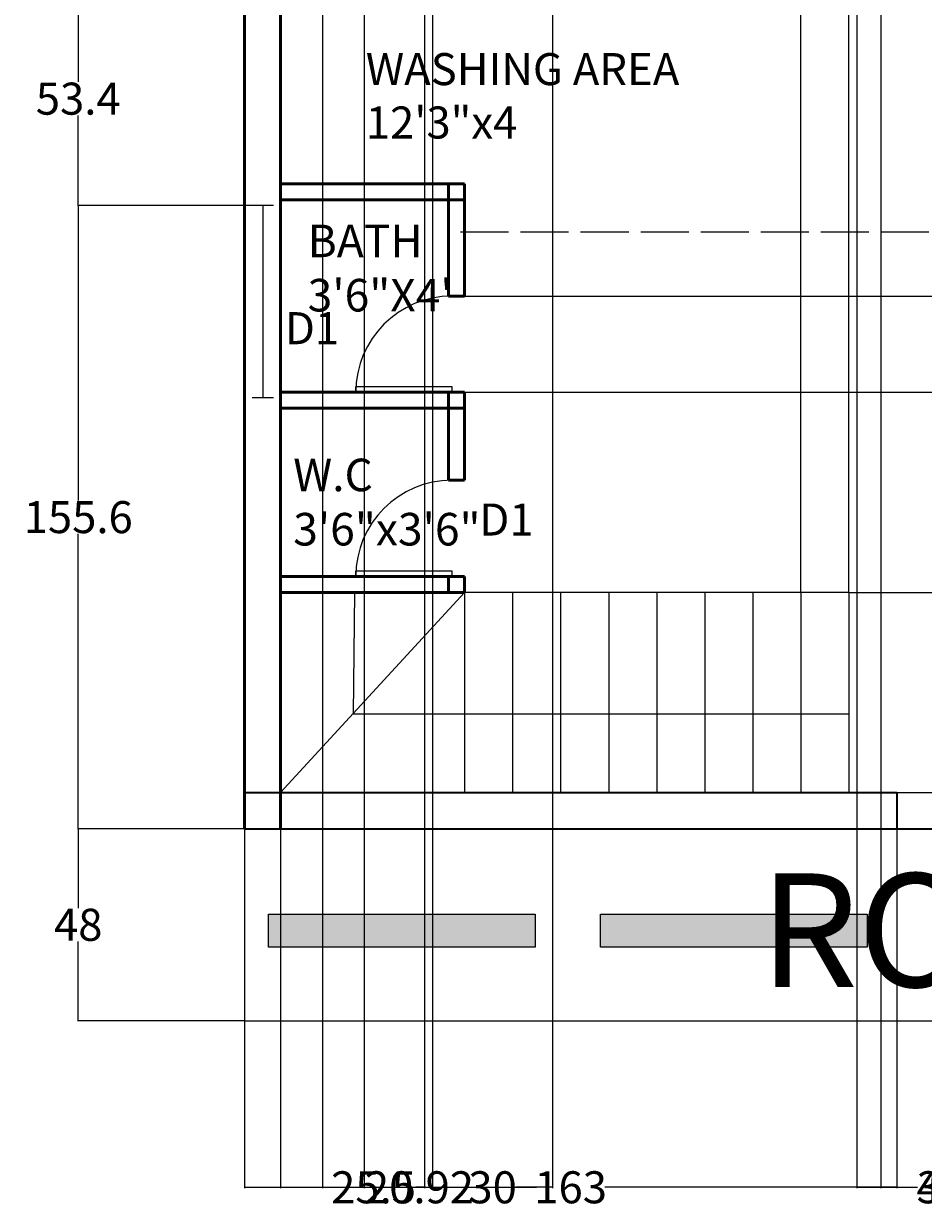
# Model space of a CAD drawing. Units: inches. Extents: x 3004 to 3478, y -798 to 114.
# Tile 1 of 5: x 3007 to 3232, y -798 to -503. Entities that reach past the tile are written whole.
import ezdxf

# ---------------------------------------------------------------- set-up
doc = ezdxf.new("R2010")
doc.units = ezdxf.units.IN
doc.header["$MEASUREMENT"] = 0
doc.linetypes.add('ACAD_ISO02W100', pattern=[15, 12, -3])
for name, color, linetype, lineweight in [('A-ANNO-DIMS', 2, 'Continuous', 18), ('A-ANNO-TEXT', 7, 'Continuous', 18), ('A-AREA-IDEN', 7, 'Continuous', 18), ('A-DOOR', 4, 'Continuous', 25), ('A-FLOR-OVHD', 8, 'ACAD_ISO02W100', 18), ('A-FLOR-STRS', 7, 'Continuous', 25), ('A-GLAZ', 4, 'Continuous', 25), ('A-WALL', 7, 'Continuous', 50), ('A-WALL-SITE', 7, 'Continuous', 35), ('C-ROAD', 8, 'Continuous', 25), ('C-ROAD-MARK', 8, 'Continuous', 18), ('C-ROAD-PATT', 8, 'Continuous', 13)]:
    doc.layers.add(name, color=color, linetype=linetype, lineweight=lineweight)
doc.styles.get("Standard").update_dxf_attribs({"font": 'arial.ttf', "height": 8})
doc.dimstyles.get("Standard").update_dxf_attribs({"dimtxt": 0.18, "dimasz": 0.18, "dimexe": 0.18, "dimexo": 0.0625, "dimgap": 0.09, "dimtad": 0, "dimtih": 1, "dimtoh": 1, "dimzin": 0, "dimdsep": 46, "dimlunit": 4, "dimtxsty": 'Standard', "dimcen": 0.09, "dimadec": 0, "dimazin": 0, "dimtfac": 1, "dimtofl": 0, "dimtmove": 0, "dimatfit": 3, "dimfxl": 1, "dimtolj": 1, "dimtzin": 0, "dimarcsym": 0})

# ---------------------------------------------------------------- blocks, each defined once
blk = doc.blocks.new('*U19')
for p, q in [((0, 0), (0, -100)), ((750, 0), (750, -100))]:
    blk.add_line(p, q)
blk.add_lwpolyline([(0, 0), (0, 750), (43.75, 750), (43.75, 0)], close=True)
blk.add_arc((0, 0), 750, 0, 90)
blk = doc.blocks.new('Window - Imperial')
for p, q in [((0, 4), (0, 0)), ((36, 4), (36, 0)), ((0, 2), (36, 2))]:
    blk.add_line(p, q)
blk = doc.blocks.new('*D40')
at = {"layer": 'A-ANNO-DIMS', "color": 0, "lineweight": -2, "transparency": 16777216}
for p, q in [((3064.06, -548.08), (3020.48, -548.08)), ((3020.66, -548.26), (3020.66, -621.71)), ((3020.66, -703.5), (3020.66, -630.05)), ((3062.15, -703.68), (3020.48, -703.68))]:
    blk.add_line(p, q, dxfattribs=at)
at = {"layer": 'A-ANNO-DIMS', "color": 0, "transparency": 16777216}
for points in [[(3020.63, -548.26), (3020.69, -548.26), (3020.66, -548.08)], [(3020.63, -703.5), (3020.69, -703.5), (3020.66, -703.68)]]:
    blk.add_solid(points, dxfattribs=at)
at = {"layer": 'Defpoints', "color": 0, "transparency": 16777216}
for p in [(3064.12, -548.08), (3020.66, -703.68), (3062.21, -703.68)]:
    blk.add_point(p, dxfattribs=at)
at = {"layer": 'A-ANNO-DIMS', "color": 0, "transparency": 16777216, "insert": (3020.66, -625.88), "char_height": 8, "attachment_point": 5}
blk.add_mtext('\\A1;155.6', dxfattribs=at)
blk = doc.blocks.new('*D41')
at = {"layer": 'A-ANNO-DIMS', "color": 0, "lineweight": -2, "transparency": 16777216}
for p, q in [((3062.15, -703.68), (3020.48, -703.68)), ((3020.66, -703.86), (3020.66, -723.5)), ((3020.66, -751.5), (3020.66, -731.85)), ((3062.15, -751.68), (3020.48, -751.68))]:
    blk.add_line(p, q, dxfattribs=at)
at = {"layer": 'A-ANNO-DIMS', "color": 0, "transparency": 16777216}
for points in [[(3020.63, -703.86), (3020.69, -703.86), (3020.66, -703.68)], [(3020.63, -751.5), (3020.69, -751.5), (3020.66, -751.68)]]:
    blk.add_solid(points, dxfattribs=at)
at = {"layer": 'Defpoints', "color": 0, "transparency": 16777216}
for p in [(3062.21, -703.68), (3020.66, -751.68), (3062.21, -751.68)]:
    blk.add_point(p, dxfattribs=at)
at = {"layer": 'A-ANNO-DIMS', "color": 0, "transparency": 16777216, "insert": (3020.66, -727.68), "char_height": 8, "attachment_point": 5}
blk.add_mtext('\\A1;48', dxfattribs=at)
blk = doc.blocks.new('*D42')
at = {"layer": 'A-ANNO-DIMS', "color": 0, "lineweight": -2, "transparency": 16777216}
for p, q in [((3062.21, -703.74), (3062.21, -793.41)), ((3225.21, -703.74), (3225.21, -793.41)), ((3062.39, -793.23), (3135.16, -793.23)), ((3225.03, -793.23), (3152.26, -793.23))]:
    blk.add_line(p, q, dxfattribs=at)
at = {"layer": 'A-ANNO-DIMS', "color": 0, "transparency": 16777216}
for points in [[(3062.39, -793.2), (3062.39, -793.26), (3062.21, -793.23)], [(3225.03, -793.2), (3225.03, -793.26), (3225.21, -793.23)]]:
    blk.add_solid(points, dxfattribs=at)
at = {"layer": 'Defpoints', "color": 0, "transparency": 16777216}
for p in [(3062.21, -703.68), (3225.21, -703.68), (3225.21, -793.23)]:
    blk.add_point(p, dxfattribs=at)
at = {"layer": 'A-ANNO-DIMS', "color": 0, "transparency": 16777216, "insert": (3143.71, -793.23), "char_height": 8, "attachment_point": 5}
blk.add_mtext('\\A1;163', dxfattribs=at)
blk = doc.blocks.new('*D52')
at = {"layer": 'A-ANNO-DIMS', "color": 0, "lineweight": -2, "transparency": 16777216}
for p, q in [((3071.15, -494.68), (3020.48, -494.68)), ((3020.66, -494.86), (3020.66, -517.2)), ((3020.66, -547.9), (3020.66, -525.56)), ((3064.06, -548.08), (3020.48, -548.08))]:
    blk.add_line(p, q, dxfattribs=at)
at = {"layer": 'A-ANNO-DIMS', "color": 0, "transparency": 16777216}
for points in [[(3020.63, -494.86), (3020.69, -494.86), (3020.66, -494.68)], [(3020.63, -547.9), (3020.69, -547.9), (3020.66, -548.08)]]:
    blk.add_solid(points, dxfattribs=at)
at = {"layer": 'Defpoints', "color": 0, "transparency": 16777216}
for p in [(3071.21, -494.68), (3020.66, -548.08), (3064.12, -548.08)]:
    blk.add_point(p, dxfattribs=at)
at = {"layer": 'A-ANNO-DIMS', "color": 0, "transparency": 16777216, "insert": (3020.66, -521.38), "char_height": 8, "attachment_point": 5}
blk.add_mtext('\\A1;53.4', dxfattribs=at)
blk = doc.blocks.new('*D53')
at = {"layer": 'A-ANNO-DIMS', "color": 0, "lineweight": -2, "transparency": 16777216}
for p, q in [((3092.13, 11.22), (3092.13, -793.41)), ((3071.21, 7.26), (3071.21, -793.41)), ((3071.39, -793.23), (3091.95, -793.23)), ((3092.13, -793.23), (3092.31, -793.23))]:
    blk.add_line(p, q, dxfattribs=at)
at = {"layer": 'A-ANNO-DIMS', "color": 0, "transparency": 16777216}
for points in [[(3071.39, -793.2), (3071.39, -793.26), (3071.21, -793.23)], [(3091.95, -793.2), (3091.95, -793.26), (3092.13, -793.23)]]:
    blk.add_solid(points, dxfattribs=at)
at = {"layer": 'Defpoints', "color": 0, "transparency": 16777216}
for p in [(3092.13, 11.28), (3071.21, 7.32), (3092.13, -793.23)]:
    blk.add_point(p, dxfattribs=at)
at = {"layer": 'A-ANNO-DIMS', "color": 0, "transparency": 16777216, "insert": (3105.93, -793.23), "char_height": 8, "attachment_point": 5}
blk.add_mtext('\\A1;20.92', dxfattribs=at)
blk = doc.blocks.new('*D56')
at = {"layer": 'A-ANNO-DIMS', "color": 0, "lineweight": -2, "transparency": 16777216}
for p, q in [((3213.27, -644.68), (3463.94, -644.68)), ((3463.76, -644.86), (3463.76, -665.5)), ((3463.76, -694.5), (3463.76, -673.85)), ((3213.27, -694.68), (3463.94, -694.68))]:
    blk.add_line(p, q, dxfattribs=at)
at = {"layer": 'A-ANNO-DIMS', "color": 0, "transparency": 16777216}
for points in [[(3463.73, -644.86), (3463.79, -644.86), (3463.76, -644.68)], [(3463.73, -694.5), (3463.79, -694.5), (3463.76, -694.68)]]:
    blk.add_solid(points, dxfattribs=at)
at = {"layer": 'Defpoints', "color": 0, "transparency": 16777216}
for p in [(3213.21, -644.68), (3213.21, -694.68), (3463.76, -694.68)]:
    blk.add_point(p, dxfattribs=at)
at = {"layer": 'A-ANNO-DIMS', "color": 0, "transparency": 16777216, "insert": (3463.76, -669.68), "char_height": 8, "attachment_point": 5}
blk.add_mtext('\\A1;50', dxfattribs=at)
blk = doc.blocks.new('*D57')
at = {"layer": 'A-ANNO-DIMS', "color": 0, "lineweight": -2, "transparency": 16777216}
for p, q in [((3201.21, -644.62), (3201.21, 109.05)), ((3201.39, 108.87), (3201.81, 108.87)), ((3213.03, 108.87), (3212.61, 108.87)), ((3213.21, -644.62), (3213.21, 109.05))]:
    blk.add_line(p, q, dxfattribs=at)
at = {"layer": 'A-ANNO-DIMS', "color": 0, "transparency": 16777216}
for points in [[(3201.39, 108.9), (3201.39, 108.84), (3201.21, 108.87)], [(3213.03, 108.9), (3213.03, 108.84), (3213.21, 108.87)]]:
    blk.add_solid(points, dxfattribs=at)
at = {"layer": 'Defpoints', "color": 0, "transparency": 16777216}
for p in [(3213.21, 108.87), (3201.21, -644.68), (3213.21, -644.68)]:
    blk.add_point(p, dxfattribs=at)
at = {"layer": 'A-ANNO-DIMS', "color": 0, "transparency": 16777216, "insert": (3207.21, 108.87), "char_height": 8, "attachment_point": 5}
blk.add_mtext('\\A1;12', dxfattribs=at)
blk = doc.blocks.new('*D58')
at = {"layer": 'A-ANNO-DIMS', "color": 0, "lineweight": -2, "transparency": 16777216}
for p, q in [((3117.27, -570.68), (3463.94, -570.68)), ((3463.76, -570.86), (3463.76, -578.57)), ((3463.76, -594.5), (3463.76, -586.78)), ((3117.27, -594.68), (3463.94, -594.68))]:
    blk.add_line(p, q, dxfattribs=at)
at = {"layer": 'A-ANNO-DIMS', "color": 0, "transparency": 16777216}
for points in [[(3463.73, -570.86), (3463.79, -570.86), (3463.76, -570.68)], [(3463.73, -594.5), (3463.79, -594.5), (3463.76, -594.68)]]:
    blk.add_solid(points, dxfattribs=at)
at = {"layer": 'Defpoints', "color": 0, "transparency": 16777216}
for p in [(3117.21, -570.68), (3117.21, -594.68), (3463.76, -594.68)]:
    blk.add_point(p, dxfattribs=at)
at = {"layer": 'A-ANNO-DIMS', "color": 0, "transparency": 16777216, "insert": (3463.76, -582.68), "char_height": 8, "attachment_point": 5}
blk.add_mtext('\\A1;24', dxfattribs=at)
blk = doc.blocks.new('*D62')
at = {"layer": 'A-ANNO-DIMS', "color": 0, "lineweight": -2, "transparency": 16777216}
for p, q in [((3081.71, -334.74), (3081.71, -793.41)), ((3107.21, -334.74), (3107.21, -793.41)), ((3081.89, -793.23), (3083.88, -793.23)), ((3107.03, -793.23), (3105.04, -793.23))]:
    blk.add_line(p, q, dxfattribs=at)
at = {"layer": 'A-ANNO-DIMS', "color": 0, "transparency": 16777216}
for points in [[(3081.89, -793.2), (3081.89, -793.26), (3081.71, -793.23)], [(3107.03, -793.2), (3107.03, -793.26), (3107.21, -793.23)]]:
    blk.add_solid(points, dxfattribs=at)
at = {"layer": 'Defpoints', "color": 0, "transparency": 16777216}
for p in [(3081.71, -334.68), (3107.21, -334.68), (3107.21, -793.23)]:
    blk.add_point(p, dxfattribs=at)
at = {"layer": 'A-ANNO-DIMS', "color": 0, "transparency": 16777216, "insert": (3094.46, -793.23), "char_height": 8, "attachment_point": 5}
blk.add_mtext('\\A1;25.5', dxfattribs=at)
blk = doc.blocks.new('*D63')
at = {"layer": 'A-ANNO-DIMS', "color": 0, "lineweight": -2, "transparency": 16777216}
for p, q in [((3221.21, -46.74), (3221.21, -793.41)), ((3251.21, -46.74), (3251.21, -793.41)), ((3221.39, -793.23), (3230.41, -793.23)), ((3251.03, -793.23), (3242.01, -793.23))]:
    blk.add_line(p, q, dxfattribs=at)
at = {"layer": 'A-ANNO-DIMS', "color": 0, "transparency": 16777216}
for points in [[(3221.39, -793.2), (3221.39, -793.26), (3221.21, -793.23)], [(3251.03, -793.2), (3251.03, -793.26), (3251.21, -793.23)]]:
    blk.add_solid(points, dxfattribs=at)
at = {"layer": 'Defpoints', "color": 0, "transparency": 16777216}
for p in [(3221.21, -46.68), (3251.21, -46.68), (3251.21, -793.23)]:
    blk.add_point(p, dxfattribs=at)
at = {"layer": 'A-ANNO-DIMS', "color": 0, "transparency": 16777216, "insert": (3236.21, -793.23), "char_height": 8, "attachment_point": 5}
blk.add_mtext('\\A1;30', dxfattribs=at)
blk = doc.blocks.new('*D64')
at = {"layer": 'A-ANNO-DIMS', "color": 0, "lineweight": -2, "transparency": 16777216}
for p, q in [((3215.21, -190.74), (3215.21, -793.41)), ((3257.21, -220.74), (3257.21, -793.41)), ((3215.39, -793.23), (3230.27, -793.23)), ((3257.03, -793.23), (3242.15, -793.23))]:
    blk.add_line(p, q, dxfattribs=at)
at = {"layer": 'A-ANNO-DIMS', "color": 0, "transparency": 16777216}
for points in [[(3215.39, -793.2), (3215.39, -793.26), (3215.21, -793.23)], [(3257.03, -793.2), (3257.03, -793.26), (3257.21, -793.23)]]:
    blk.add_solid(points, dxfattribs=at)
at = {"layer": 'Defpoints', "color": 0, "transparency": 16777216}
for p in [(3215.21, -190.68), (3257.21, -220.68), (3257.21, -793.23)]:
    blk.add_point(p, dxfattribs=at)
at = {"layer": 'A-ANNO-DIMS', "color": 0, "transparency": 16777216, "insert": (3236.21, -793.23), "char_height": 8, "attachment_point": 5}
blk.add_mtext('\\A1;42', dxfattribs=at)
blk = doc.blocks.new('*D65')
at = {"layer": 'A-ANNO-DIMS', "color": 0, "lineweight": -2, "transparency": 16777216}
for p, q in [((3109.21, -46.74), (3109.21, -793.41)), ((3139.21, -46.74), (3139.21, -793.41)), ((3109.39, -793.23), (3118.41, -793.23)), ((3139.03, -793.23), (3130.01, -793.23))]:
    blk.add_line(p, q, dxfattribs=at)
at = {"layer": 'A-ANNO-DIMS', "color": 0, "transparency": 16777216}
for points in [[(3109.39, -793.2), (3109.39, -793.26), (3109.21, -793.23)], [(3139.03, -793.2), (3139.03, -793.26), (3139.21, -793.23)]]:
    blk.add_solid(points, dxfattribs=at)
at = {"layer": 'Defpoints', "color": 0, "transparency": 16777216}
for p in [(3109.21, -46.68), (3139.21, -46.68), (3139.21, -793.23)]:
    blk.add_point(p, dxfattribs=at)
at = {"layer": 'A-ANNO-DIMS', "color": 0, "transparency": 16777216, "insert": (3124.21, -793.23), "char_height": 8, "attachment_point": 5}
blk.add_mtext('\\A1;30', dxfattribs=at)

msp = doc.modelspace()

# ---------------------------------------------------------------- hatches: boundary and pattern name
at = {"layer": 'C-ROAD-PATT'}
h = msp.add_hatch(color=256, dxfattribs=at)
h.dxf.hatch_style = 1
h.paths.add_polyline_path([(3134.8245, -725.0263), (3068.2428, -725.0263), (3068.2428, -733.2952), (3134.8245, -733.2952)])
h.paths.add_polyline_path([(3217.7696, -725.0263), (3151.1878, -725.0263), (3151.1878, -733.2952), (3217.7696, -733.2952)])
h.paths.add_polyline_path([(3180.7889, -759.1898), (3309.3973, -759.1898), (3309.3973, -700.7648), (3180.7889, -700.7648)], flags=9)
h = msp.add_hatch(color=256, dxfattribs=at)
h.dxf.hatch_style = 1
h.paths.add_polyline_path([(3406.0421, -725.0263), (3339.4603, -725.0263), (3339.4603, -733.2952), (3406.0421, -733.2952)])
h.paths.add_polyline_path([(3332.0926, -725.0263), (3265.5108, -725.0263), (3265.5108, -733.2952), (3332.0926, -733.2952)])
h.paths.add_polyline_path([(3180.7889, -759.1898), (3309.3973, -759.1898), (3309.3973, -700.7648), (3180.7889, -700.7648)], flags=9)

# ---------------------------------------------------------------- linework, layer by layer
at = {"layer": 'A-FLOR-OVHD'}
msp.add_line((3413.2113, -554.6779), (3113.2113, -554.6779), dxfattribs=at)
at = {"layer": 'A-FLOR-STRS'}
for p, q in [((3117.2113, -644.6779), (3071.2113, -694.6779)), ((3089.7113, -644.6779), (3089.3381, -674.9749)), ((3117.2113, -644.6779), (3117.2113, -694.6779)), ((3213.2113, -644.6779), (3117.2113, -644.6779)), ((3129.2113, -644.6779), (3129.2113, -694.6779)), ((3141.2113, -644.6779), (3141.2113, -694.6779)), ((3153.2113, -644.6779), (3153.2113, -694.6779)), ((3165.2113, -644.6779), (3165.2113, -694.6779)), ((3177.2113, -644.6779), (3177.2113, -694.6779)), ((3189.2113, -644.6779), (3189.2113, -694.6779)), ((3201.2113, -644.6779), (3201.2113, -694.6779)), ((3213.2113, -644.6779), (3213.2113, -694.6779)), ((3089.3381, -674.9749), (3213.2113, -674.9749))]:
    msp.add_line(p, q, dxfattribs=at)
at = {"layer": 'A-WALL'}
for p, q in [((3062.2113, 16.3221), (3062.2113, -703.6779)), ((3071.2113, 7.3221), (3071.2113, -703.6779)), ((3117.2113, -542.6779), (3071.2113, -542.6779)), ((3113.2113, -542.6779), (3113.2113, -570.6779)), ((3117.2113, -542.6779), (3117.2113, -570.6779)), ((3117.2113, -546.6779), (3071.2113, -546.6779)), ((3113.2113, -570.6779), (3117.2113, -570.6779)), ((3117.2113, -594.6779), (3071.2113, -594.6779)), ((3113.2113, -594.6779), (3113.2113, -616.6779)), ((3117.2113, -594.6779), (3117.2113, -616.6779)), ((3117.2113, -598.6779), (3071.2113, -598.6779)), ((3117.2113, -616.6779), (3113.2113, -616.6779)), ((3117.2113, -640.6779), (3071.2113, -640.6779)), ((3113.2113, -640.6779), (3113.2113, -644.6779)), ((3117.2113, -640.6779), (3117.2113, -644.6779)), ((3117.2113, -644.6779), (3071.2113, -644.6779))]:
    msp.add_line(p, q, dxfattribs=at)
at = {"layer": 'A-WALL-SITE'}
for p, q in [((3062.2113, -694.6779), (3225.2113, -694.6779)), ((3213.2113, -694.6779), (3225.2113, -694.6779)), ((3225.2113, -694.6779), (3225.2113, -703.6779)), ((3062.2113, -703.6779), (3422.2113, -703.6779))]:
    msp.add_line(p, q, dxfattribs=at)
at = {"layer": 'C-ROAD'}
for p, q in [((3062.2113, -703.6779), (3062.2113, -751.6779)), ((3062.2113, -751.6779), (3422.2113, -751.6779))]:
    msp.add_line(p, q, dxfattribs=at)
at = {"layer": 'C-ROAD-MARK'}
for points in [[(3068.2428, -725.0263), (3134.8245, -725.0263), (3134.8245, -733.2952), (3068.2428, -733.2952)], [(3151.1878, -725.0263), (3217.7696, -725.0263), (3217.7696, -733.2952), (3151.1878, -733.2952)]]:
    msp.add_lwpolyline(points, close=True, dxfattribs=at)

# ---------------------------------------------------------------- block references
at = {"layer": 'A-DOOR', "xscale": 0.0319999999999999, "yscale": 0.0319999999999999, "zscale": 0.0319999999999999, "rotation": 90}
for p in [(3114.0113, -594.6779), (3114.0113, -640.6779)]:
    msp.add_blockref('*U19', p, dxfattribs=at)
at = {"layer": 'A-GLAZ', "xscale": 1.333333333333333, "yscale": 1.333333333333333, "zscale": 1.333333333333333, "rotation": 270}
msp.add_blockref('Window - Imperial', (3064.1176, -548.0828), dxfattribs=at)

# ---------------------------------------------------------------- texts
at = {"layer": 'A-ANNO-TEXT', "attachment_point": 1}
for s, width, gutter_width, insert, char_height in [('D1', 22.083935, 40, (3072.302, -574.6953), 8), ('D1', 22.083935, 40, (3120.8932, -622.4837), 8), ('ROAD', 577.293337, 141.7594, (3190.9905, -714.8537), 28.35188)]:
    msp.add_mtext_dynamic_manual_height_columns(s, width=width, gutter_width=gutter_width, heights=[0], dxfattribs=dict(at, insert=insert, char_height=char_height))
at = {"layer": 'A-AREA-IDEN', "attachment_point": 1}
for s, width, gutter_width, insert, char_height in [('WASHING AREA\\P12\'3"x4', 228.23715, 40, (3092.523, -510.0002), 8), ('BATH\\P3\'6"X4\'', 231.882133, 40.6388, (3077.9929, -552.8439), 8.12776), ('W.C\\P3\'6"x3\'6"', 228.23715, 40, (3074.3867, -611.281), 8.12776)]:
    msp.add_mtext_dynamic_manual_height_columns(s, width=width, gutter_width=gutter_width, heights=[0], dxfattribs=dict(at, insert=insert, char_height=char_height))

# ---------------------------------------------------------------- dimensions: what is measured, and where the dimension line sits
at = {"layer": 'A-ANNO-DIMS'}
for base, p1, p2, override, picture, middle in [((3213.2113, 108.8721), (3201.2113, -644.6779), (3213.2113, -644.6779), {"dimdec": 0, "dimlfac": 1, "dimrnd": 0, "dimzin": 0, "dimdsep": 46, "dimlunit": 2}, '*D57', (3207.2113, 108.8721)), ((3092.1316, -793.2279), (3071.2113, 7.3221), (3092.1316, 11.284), {"dimdec": 2, "dimlfac": 1, "dimrnd": 0, "dimzin": 0, "dimdsep": 46, "dimlunit": 2}, '*D53', (3105.9268, -793.2279)), ((3139.2113, -793.2279), (3109.2113, -46.6779), (3139.2113, -46.6779), {"dimdec": 0, "dimlfac": 1, "dimrnd": 0, "dimzin": 0, "dimdsep": 46, "dimlunit": 2}, '*D65', (3124.2113, -793.2279)), ((3251.2113, -793.2279), (3221.2113, -46.6779), (3251.2113, -46.6779), {"dimdec": 0, "dimlfac": 1, "dimrnd": 0, "dimzin": 0, "dimdsep": 46, "dimlunit": 2}, '*D63', (3236.2113, -793.2279)), ((3257.2113, -793.2279), (3215.2113, -190.6779), (3257.2113, -220.6779), {"dimdec": 0, "dimlfac": 1, "dimrnd": 0, "dimzin": 0, "dimdsep": 46, "dimlunit": 2}, '*D64', (3236.2113, -793.2279)), ((3107.2113, -793.2279), (3081.7115, -334.6779), (3107.2113, -334.6779), {"dimdec": 1, "dimlfac": 1, "dimrnd": 0, "dimzin": 0, "dimdsep": 46, "dimlunit": 2}, '*D62', (3094.4614, -793.2279)), ((3225.2113, -793.2279), (3062.2113, -703.6779), (3225.2113, -703.6779), {"dimdec": 0, "dimlfac": 1, "dimrnd": 0, "dimzin": 0, "dimdsep": 46, "dimlunit": 2}, '*D42', (3143.7113, -793.2279))]:
    dim = msp.add_linear_dim(base=base, p1=p1, p2=p2, dimstyle='Standard', override=override, dxfattribs=at)
    dim.commit()
    dim.dimension.update_dxf_attribs({"geometry": picture, "text_midpoint": middle})
for base, p1, p2, override, picture, middle in [((3020.6613, -548.0828), (3071.2113, -494.6779), (3064.1176, -548.0828), {"dimdec": 1, "dimlfac": 1, "dimrnd": 0, "dimzin": 0, "dimdsep": 46, "dimlunit": 2}, '*D52', (3020.6613, -521.3803)), ((3020.6613, -703.6779), (3064.1176, -548.0828), (3062.2113, -703.6779), {"dimdec": 1, "dimlfac": 1, "dimrnd": 0, "dimzin": 0, "dimdsep": 46, "dimlunit": 2}, '*D40', (3020.6613, -625.8803)), ((3463.7613, -594.6779), (3117.2113, -570.6779), (3117.2113, -594.6779), {"dimdec": 0, "dimlfac": 1, "dimrnd": 0, "dimzin": 0, "dimdsep": 46, "dimlunit": 2}, '*D58', (3463.7613, -582.6779)), ((3463.7613, -694.6779), (3213.2113, -644.6779), (3213.2113, -694.6779), {"dimdec": 0, "dimlfac": 1, "dimrnd": 0, "dimzin": 0, "dimdsep": 46, "dimlunit": 2}, '*D56', (3463.7613, -669.6779)), ((3020.6613, -751.6779), (3062.2113, -703.6779), (3062.2113, -751.6779), {"dimdec": 0, "dimlfac": 1, "dimrnd": 0, "dimzin": 0, "dimdsep": 46, "dimlunit": 2}, '*D41', (3020.6613, -727.6779))]:
    dim = msp.add_linear_dim(base=base, p1=p1, p2=p2, angle=90, dimstyle='Standard', override=override, dxfattribs=at)
    dim.commit()
    dim.dimension.update_dxf_attribs({"geometry": picture, "text_midpoint": middle})

doc.saveas('drawing.dxf')
